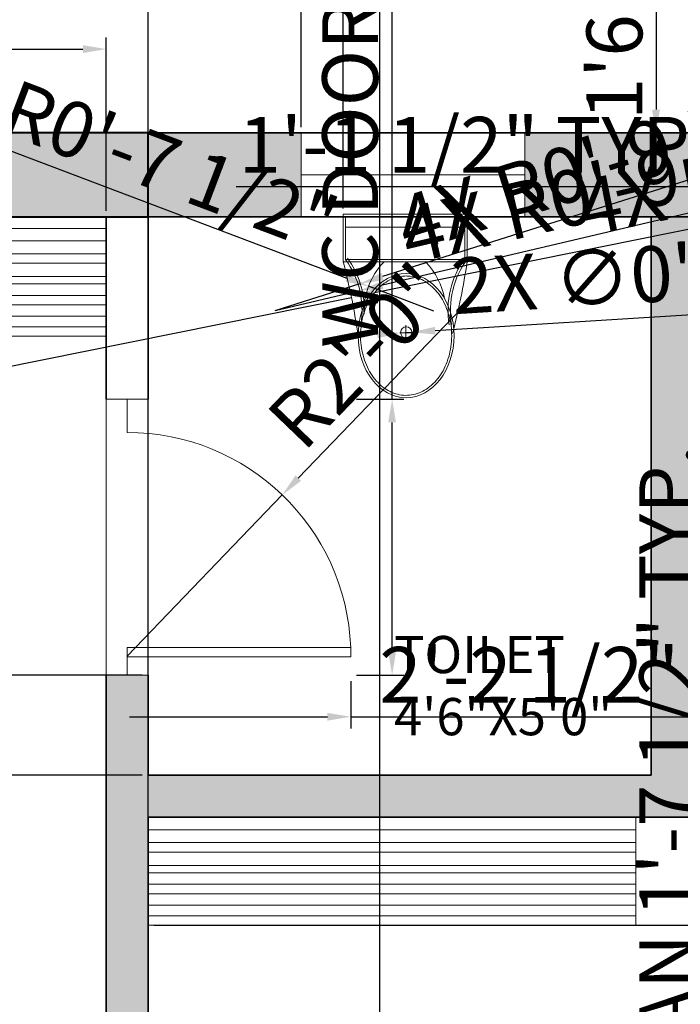
# Model space of a CAD drawing. Units: inches. Extents: x 2656 to 9931, y 1941 to 3068.
# Tile 22 of 46: x 2863 to 2934, y 2530 to 2636. Entities that reach past the tile are written whole.
import ezdxf

# ---------------------------------------------------------------- set-up
doc = ezdxf.new("R2010")
doc.units = ezdxf.units.IN
for name, color, linetype, lineweight in [('A-ANNO-DIMS', 2, 'Continuous', 18), ('A-AREA-IDEN', 7, 'Continuous', 18), ('A-COLS', 7, 'Continuous', 40), ('A-COLS-PATT', 146, 'Continuous', 13), ('A-DOOR', 3, 'Continuous', 18), ('A-FLOR-CASE', 32, 'Continuous', 18), ('A-FLOR-FIXT', 9, 'Continuous', 18), ('A-GLAZ', 4, 'Continuous', 18), ('A-WALL', 7, 'Continuous', 35), ('A-WALL-PATT', 251, 'Continuous', 13)]:
    doc.layers.add(name, color=color, linetype=linetype, lineweight=lineweight)
doc.styles.get("Standard").update_dxf_attribs({"font": 'arial.ttf'})
doc.dimstyles.new('ISO-25', dxfattribs={"dimtxt": 6, "dimasz": 2.5, "dimexe": 1.25, "dimexo": 0.625, "dimtad": 1, "dimdec": 0, "dimlunit": 3, "dimtxsty": 'Standard', "dimcen": 2.5, "dimadec": 0, "dimazin": 0, "dimtfac": 1, "dimtdec": 0, "dimtmove": 0, "dimatfit": 3, "dimfxl": 1, "dimarcsym": 0})

# ---------------------------------------------------------------- blocks, each defined once
blk = doc.blocks.new('*D2')
at = {"layer": 'A-ANNO-DIMS', "color": 0, "lineweight": -2, "transparency": 16777216}
for p, q in [((2931.82, 2641.6), (2932.44, 2641.6)), ((2931.19, 2639.1), (2931.19, 2626.1)), ((2931.82, 2623.6), (2932.44, 2623.6))]:
    blk.add_line(p, q, dxfattribs=at)
at = {"layer": 'A-ANNO-DIMS', "color": 0, "transparency": 16777216}
for points in [[(2930.77, 2639.1), (2931.61, 2639.1), (2931.19, 2641.6)], [(2930.77, 2626.1), (2931.61, 2626.1), (2931.19, 2623.6)]]:
    blk.add_solid(points, dxfattribs=at)
at = {"layer": 'Defpoints', "color": 0, "transparency": 16777216}
for p in [(2931.19, 2641.6), (2931.19, 2623.6), (2931.19, 2623.6)]:
    blk.add_point(p, dxfattribs=at)
at = {"layer": 'A-ANNO-DIMS', "color": 0, "transparency": 16777216, "insert": (2927.5, 2632.6), "char_height": 6, "attachment_point": 5, "rotation": 90}
blk.add_mtext('1\'6"', dxfattribs=at)
blk = doc.blocks.new('A$C31115884')
for p, q in [((283.1, 497.7), (223.4, 497.7)), ((257.5, 466.4), (257.5, 523.2)), ((0, 200), (0, 0)), ((520, 200), (0, 200)), ((10, 190), (10, 10)), ((510, 190), (10, 190)), ((510, 10), (510, 190)), ((520, 0), (520, 200)), ((510, 54.5), (0, 54.5)), ((10, 10), (510, 10)), ((0, 0), (520, 0))]:
    blk.add_line(p, q)
blk.add_circle((255.6, 496.4), 23.6)
for centre, radius, start, end in [((2777.7, -204.6), 2807, 165.4549, 171.7133), ((3237, 905), 2807, 188.2867, 194.5451), ((-294.5, 403.3), 364.7, 324.2091, 9.3499), ((-294.5, 403.3), 374.7, 324.2091, 9.3499), ((805.8, 403.3), 364.7, 170.6501, 215.7909), ((139.5, 406.2), 293.5, 315.8436, 2.6563), ((805.8, 403.3), 374.7, 179.2036, 215.7909), ((383.6, 406.2), 293.5, 190.2774, 224.1564)]:
    blk.add_arc(centre, radius, start, end)
blk.add_ellipse((256.2, 509.9), major_axis=(0, -260.7), ratio=0.772727)
blk.add_open_spline([(256.2, 259.2), (263.1, 259.2), (270, 259.7), (287.8, 262.3), (298.7, 265.1), (319.9, 273.1), (330.2, 278.4), (350.1, 291.1), (359.7, 298.7), (377.7, 315.9), (386.2, 325.5), (401.7, 346.6), (408.8, 358.1), (421.3, 382.5), (426.8, 395.5), (435.9, 422.4), (439.5, 436.4), (444.8, 465.1), (446.5, 479.7), (447.9, 509.2), (447.6, 524), (445, 553.3), (442.7, 567.8), (436.3, 596), (432.1, 609.7), (421.9, 636), (416, 648.6), (402.5, 672.1), (395, 683), (378.6, 703), (369.8, 712.1), (351.1, 728), (341.3, 734.8), (320.9, 746.2), (310.4, 750.7), (288.9, 757.3), (278, 759.4), (256, 761), (245, 760.6), (223.1, 757.2), (212.3, 754.3), (191.1, 746.1), (180.8, 740.7), (160.9, 727.8), (151.4, 720.1), (133.5, 702.7), (125.1, 693), (109.6, 671.7), (102.6, 660.2), (90.2, 635.7), (84.9, 622.7), (76, 595.6), (72.4, 581.6), (67.2, 552.9), (65.6, 538.2), (64.4, 508.8), (64.8, 494), (67.5, 464.7), (69.9, 450.2), (76.6, 422), (80.8, 408.3), (91.1, 382.2), (97.2, 369.7), (110.8, 346.3), (118.4, 335.4), (134.8, 315.6), (143.7, 306.7), (162.4, 290.9), (172.3, 284.2), (192.8, 273), (203.3, 268.6), (224.8, 262.2), (235.8, 260.2), (249.9, 259.3), (253, 259.2), (256.2, 259.2)], degree=3, knots=[0, 0, 0, 0, 0.110105, 0.110105, 0.285049, 0.285049, 0.459994, 0.459994, 0.634938, 0.634938, 0.809882, 0.809882, 0.984827, 0.984827, 1.159771, 1.159771, 1.334715, 1.334715, 1.50966, 1.50966, 1.684604, 1.684604, 1.859549, 1.859549, 2.034493, 2.034493, 2.209437, 2.209437, 2.384382, 2.384382, 2.559326, 2.559326, 2.73427, 2.73427, 2.909215, 2.909215, 3.084159, 3.084159, 3.259103, 3.259103, 3.434048, 3.434048, 3.608992, 3.608992, 3.783936, 3.783936, 3.958881, 3.958881, 4.133825, 4.133825, 4.30877, 4.30877, 4.483714, 4.483714, 4.658658, 4.658658, 4.833603, 4.833603, 5.008547, 5.008547, 5.183491, 5.183491, 5.358436, 5.358436, 5.53338, 5.53338, 5.708324, 5.708324, 5.883269, 5.883269, 6.058213, 6.058213, 6.233158, 6.233158, 6.283185, 6.283185, 6.283185, 6.283185])
blk = doc.blocks.new('DOOR-WC-SIDE')
for p, q in [((-0.04, 29.7), (-0.04, 0.04)), ((2.21, 29.7), (2.21, 28.12)), ((2.21, 28.12), (2.21, 26.12)), ((26.21, 3.04), (2.21, 3.04)), ((2.21, 3.04), (2.21, 2.04)), ((26.21, 2.04), (26.21, 3.04)), ((2.21, 0.04), (2.21, 2.04)), ((2.21, 2.04), (2.21, 2.04)), ((2.21, 2.04), (26.21, 2.04))]:
    blk.add_line(p, q)
blk.add_arc((2.21, 2.11), 24.02, 2.2244, 90)
blk = doc.blocks.new('WIN-VENT-24IN')
for p, q in [((23.99, 0), (23.99, 4.5)), ((-0.01, 0), (23.99, 0))]:
    blk.add_line(p, q)
blk = doc.blocks.new('WARDROBE-LONG')
for p, q in [((34.19, 12.8), (34.19, -0.03)), ((34.19, 11.55), (119.96, 11.55)), ((34.19, 10.19), (119.96, 10.19)), ((34.19, 8.82), (119.96, 8.82)), ((34.19, 7.81), (119.96, 7.81)), ((34.19, 6.39), (119.96, 6.39)), ((34.19, 5.58), (119.96, 5.58)), ((34.19, 4.35), (119.96, 4.35)), ((34.19, 3.33), (119.96, 3.33)), ((34.19, 2.12), (119.96, 2.12)), ((34.19, 2.12), (119.96, 2.12)), ((34.19, -0.03), (34.19, 0.97)), ((34.19, 0.97), (119.96, 0.97)), ((-0.04, -0.03), (119.96, -0.03))]:
    blk.add_line(p, q)
blk = doc.blocks.new('WARDROBE-SHORT')
for p, q in [((52.34, 11.6), (52.34, 0.02)), ((-0.04, 10.24), (52.34, 10.24)), ((-0.04, 8.87), (52.34, 8.87)), ((-0.04, 7.85), (52.34, 7.85)), ((-0.04, 6.43), (52.34, 6.43)), ((-0.04, 5.63), (52.34, 5.63)), ((-0.04, 4.4), (52.34, 4.4)), ((-0.04, 3.38), (52.34, 3.38)), ((-0.04, 2.17), (52.34, 2.17)), ((-0.04, 2.17), (52.34, 2.17)), ((-0.04, 1.02), (52.34, 1.02)), ((-0.04, 0.02), (52.34, 0.02))]:
    blk.add_line(p, q)
blk = doc.blocks.new('*D29')
at = {"layer": 'A-ANNO-DIMS', "color": 0, "lineweight": -2, "transparency": 16777216}
for p, q in [((2939.24, 2614.86), (2935.66, 2614.86)), ((2936.91, 2612.36), (2936.91, 2597.65)), ((2939.24, 2595.15), (2935.66, 2595.15)), ((2936.91, 2595.15), (2936.91, 2504.75))]:
    blk.add_line(p, q, dxfattribs=at)
at = {"layer": 'A-ANNO-DIMS', "color": 0, "transparency": 16777216}
for points in [[(2936.49, 2612.36), (2937.33, 2612.36), (2936.91, 2614.86)], [(2936.49, 2597.65), (2937.33, 2597.65), (2936.91, 2595.15)]]:
    blk.add_solid(points, dxfattribs=at)
at = {"layer": 'Defpoints', "color": 0, "transparency": 16777216}
for p in [(2939.87, 2614.86), (2936.91, 2595.15), (2939.87, 2595.15)]:
    blk.add_point(p, dxfattribs=at)
at = {"layer": 'A-ANNO-DIMS', "color": 0, "transparency": 16777216, "insert": (2933.18, 2548.7), "char_height": 6, "attachment_point": 5, "rotation": 90}
blk.add_mtext('WC PAN 1\'-7 1/2" TYP.', dxfattribs=at)
blk = doc.blocks.new('*D30')
at = {"layer": 'A-ANNO-DIMS', "color": 0, "lineweight": -2, "transparency": 16777216}
for p, q in [((2939.87, 2615.48), (2939.87, 2619.06)), ((2953.16, 2615.48), (2953.16, 2619.06)), ((2939.87, 2617.81), (2886.13, 2617.81)), ((2950.66, 2617.81), (2942.37, 2617.81))]:
    blk.add_line(p, q, dxfattribs=at)
at = {"layer": 'A-ANNO-DIMS', "color": 0, "transparency": 16777216}
for points in [[(2942.37, 2618.23), (2942.37, 2617.39), (2939.87, 2617.81)], [(2950.66, 2618.23), (2950.66, 2617.39), (2953.16, 2617.81)]]:
    blk.add_solid(points, dxfattribs=at)
at = {"layer": 'Defpoints', "color": 0, "transparency": 16777216}
for p in [(2939.87, 2617.81), (2939.87, 2614.86), (2953.16, 2614.86)]:
    blk.add_point(p, dxfattribs=at)
at = {"layer": 'A-ANNO-DIMS', "color": 0, "transparency": 16777216, "insert": (2911.75, 2621.54), "char_height": 6, "attachment_point": 5}
blk.add_mtext('1\'-1 1/2" TYP.', dxfattribs=at)
blk = doc.blocks.new('*D32')
at = {"layer": 'A-ANNO-DIMS', "color": 0, "lineweight": -2, "transparency": 16777216}
for p, q in [((2842.61, 2565.21), (2856.53, 2565.21)), ((2855.28, 2505.27), (2855.28, 2562.71)), ((2842.61, 2502.77), (2856.53, 2502.77))]:
    blk.add_line(p, q, dxfattribs=at)
at = {"layer": 'A-ANNO-DIMS', "color": 0, "transparency": 16777216}
for points in [[(2854.86, 2562.71), (2855.69, 2562.71), (2855.28, 2565.21)], [(2854.86, 2505.27), (2855.69, 2505.27), (2855.28, 2502.77)]]:
    blk.add_solid(points, dxfattribs=at)
at = {"layer": 'Defpoints', "color": 0, "transparency": 16777216}
for p in [(2841.98, 2565.21), (2855.28, 2565.21), (2841.98, 2502.77)]:
    blk.add_point(p, dxfattribs=at)
at = {"layer": 'A-ANNO-DIMS', "color": 0, "transparency": 16777216, "insert": (2851.55, 2533.99), "char_height": 6, "attachment_point": 5, "rotation": 90}
blk.add_mtext('5\'-2 1/2" TYP.', dxfattribs=at)
blk = doc.blocks.new('*D33')
at = {"layer": 'A-ANNO-DIMS', "color": 0, "lineweight": -2, "transparency": 16777216}
for p, q in [((2902.86, 2595), (2902.86, 2693.32)), ((2899.03, 2595), (2904.11, 2595)), ((2902.86, 2567.84), (2902.86, 2592.5)), ((2899.03, 2565.34), (2904.11, 2565.34))]:
    blk.add_line(p, q, dxfattribs=at)
at = {"layer": 'A-ANNO-DIMS', "color": 0, "transparency": 16777216}
for points in [[(2902.44, 2592.5), (2903.27, 2592.5), (2902.86, 2595)], [(2902.44, 2567.84), (2903.27, 2567.84), (2902.86, 2565.34)]]:
    blk.add_solid(points, dxfattribs=at)
at = {"layer": 'Defpoints', "color": 0, "transparency": 16777216}
for p in [(2898.41, 2595), (2902.86, 2595), (2898.41, 2565.34)]:
    blk.add_point(p, dxfattribs=at)
at = {"layer": 'A-ANNO-DIMS', "color": 0, "transparency": 16777216, "insert": (2899.13, 2645.41), "char_height": 6, "attachment_point": 5, "rotation": 90}
blk.add_mtext('WC DOOR 2\'-5 1/2" TYP.', dxfattribs=at)
blk = doc.blocks.new('*D34')
at = {"layer": 'A-ANNO-DIMS', "color": 0, "lineweight": -2, "transparency": 16777216}
for p, q in [((2872.16, 2564.71), (2872.16, 2559.64)), ((2898.41, 2564.71), (2898.41, 2559.64)), ((2874.66, 2560.89), (2895.91, 2560.89)), ((2898.41, 2560.89), (2952.81, 2560.89))]:
    blk.add_line(p, q, dxfattribs=at)
at = {"layer": 'A-ANNO-DIMS', "color": 0, "transparency": 16777216}
for points in [[(2874.66, 2561.3), (2874.66, 2560.47), (2872.16, 2560.89)], [(2895.91, 2561.3), (2895.91, 2560.47), (2898.41, 2560.89)]]:
    blk.add_solid(points, dxfattribs=at)
at = {"layer": 'Defpoints', "color": 0, "transparency": 16777216}
for p in [(2872.16, 2565.34), (2898.41, 2565.34), (2898.41, 2560.89)]:
    blk.add_point(p, dxfattribs=at)
at = {"layer": 'A-ANNO-DIMS', "color": 0, "transparency": 16777216, "insert": (2926.86, 2564.61), "char_height": 6, "attachment_point": 5}
blk.add_mtext('2\'-2 1/2" TYP.', dxfattribs=at)
blk = doc.blocks.new('*D57')
at = {"layer": 'A-ANNO-DIMS', "color": 0, "lineweight": -2, "transparency": 16777216}
for p, q in [((2752.16, 2615.23), (2752.16, 2633.85)), ((2872.16, 2615.23), (2872.16, 2633.85)), ((2754.66, 2632.6), (2869.66, 2632.6))]:
    blk.add_line(p, q, dxfattribs=at)
at = {"layer": 'A-ANNO-DIMS', "color": 0, "transparency": 16777216}
for points in [[(2754.66, 2633.02), (2754.66, 2632.18), (2752.16, 2632.6)], [(2869.66, 2633.02), (2869.66, 2632.18), (2872.16, 2632.6)]]:
    blk.add_solid(points, dxfattribs=at)
at = {"layer": 'Defpoints', "color": 0, "transparency": 16777216}
for p in [(2872.16, 2632.6), (2752.16, 2614.6), (2872.16, 2614.6)]:
    blk.add_point(p, dxfattribs=at)
at = {"layer": 'A-ANNO-DIMS', "color": 0, "transparency": 16777216, "insert": (2812.16, 2636.33), "char_height": 6, "attachment_point": 5}
blk.add_mtext('WARDROBE 10\'-0" TYP.', dxfattribs=at)
blk = doc.blocks.new('*D98')
at = {"layer": 'A-ANNO-DIMS', "color": 0, "lineweight": -2, "transparency": 16777216}
for p, q in [((2876.66, 2624.23), (2876.66, 2674.45)), ((2893.09, 2624.23), (2893.09, 2674.45)), ((2879.16, 2673.2), (2890.59, 2673.2)), ((2893.09, 2673.2), (2926.2, 2673.2))]:
    blk.add_line(p, q, dxfattribs=at)
at = {"layer": 'A-ANNO-DIMS', "color": 0, "transparency": 16777216}
for points in [[(2879.16, 2673.62), (2879.16, 2672.78), (2876.66, 2673.2)], [(2890.59, 2673.62), (2890.59, 2672.78), (2893.09, 2673.2)]]:
    blk.add_solid(points, dxfattribs=at)
at = {"layer": 'Defpoints', "color": 0, "transparency": 16777216}
for p in [(2893.09, 2673.2), (2876.66, 2623.6), (2893.09, 2623.6)]:
    blk.add_point(p, dxfattribs=at)
at = {"layer": 'A-ANNO-DIMS', "color": 0, "transparency": 16777216, "insert": (2910.89, 2676.93), "char_height": 6, "attachment_point": 5}
blk.add_mtext('1\'-4 1/2"', dxfattribs=at)
blk = doc.blocks.new('*D100')
at = {"layer": 'A-ANNO-DIMS', "color": 0, "lineweight": -2, "transparency": 16777216}
for p, q in [((2696.56, 2565.34), (2696.56, 2603.68)), ((2876.03, 2565.34), (2695.31, 2565.34)), ((2696.56, 2557.1), (2696.56, 2562.84)), ((2876.03, 2554.6), (2695.31, 2554.6))]:
    blk.add_line(p, q, dxfattribs=at)
at = {"layer": 'A-ANNO-DIMS', "color": 0, "transparency": 16777216}
for points in [[(2696.14, 2562.84), (2696.97, 2562.84), (2696.56, 2565.34)], [(2696.14, 2557.1), (2696.97, 2557.1), (2696.56, 2554.6)]]:
    blk.add_solid(points, dxfattribs=at)
at = {"layer": 'Defpoints', "color": 0, "transparency": 16777216}
for p in [(2696.56, 2565.34), (2876.66, 2565.34), (2876.66, 2554.6)]:
    blk.add_point(p, dxfattribs=at)
at = {"layer": 'A-ANNO-DIMS', "color": 0, "transparency": 16777216, "insert": (2692.83, 2585.76), "char_height": 6, "attachment_point": 5, "rotation": 90}
blk.add_mtext('0\'-10 1/2"', dxfattribs=at)
blk = doc.blocks.new('*D102')
at = {"layer": 'A-ANNO-DIMS', "color": 0, "lineweight": -2, "transparency": 16777216}
for p, q in [((2998.16, 2604.98), (2998.16, 2009.27)), ((2872.16, 2564.71), (2872.16, 2009.27)), ((2874.66, 2010.52), (2995.66, 2010.52))]:
    blk.add_line(p, q, dxfattribs=at)
at = {"layer": 'A-ANNO-DIMS', "color": 0, "transparency": 16777216}
for points in [[(2874.66, 2010.94), (2874.66, 2010.11), (2872.16, 2010.52)], [(2995.66, 2010.94), (2995.66, 2010.11), (2998.16, 2010.52)]]:
    blk.add_solid(points, dxfattribs=at)
at = {"layer": 'Defpoints', "color": 0, "transparency": 16777216}
for p in [(2998.16, 2605.6), (2872.16, 2565.34), (2998.16, 2010.52)]:
    blk.add_point(p, dxfattribs=at)
at = {"layer": 'A-ANNO-DIMS', "color": 0, "transparency": 16777216, "insert": (2935.16, 2014.21), "char_height": 6, "attachment_point": 5}
blk.add_mtext('10\'-6"', dxfattribs=at)
blk = doc.blocks.new('*D130')
at = {"layer": 'A-ANNO-DIMS', "color": 0, "lineweight": -2, "transparency": 16777216}
for p, q in [((2877.28, 2538.52), (3061.01, 2538.52)), ((3059.76, 2536.02), (3059.76, 2525.32)), ((2902.17, 2522.82), (3061.01, 2522.82)), ((3059.76, 2522.82), (3059.76, 2489.7))]:
    blk.add_line(p, q, dxfattribs=at)
at = {"layer": 'A-ANNO-DIMS', "color": 0, "transparency": 16777216}
for points in [[(3059.34, 2536.02), (3060.17, 2536.02), (3059.76, 2538.52)], [(3059.34, 2525.32), (3060.17, 2525.32), (3059.76, 2522.82)]]:
    blk.add_solid(points, dxfattribs=at)
at = {"layer": 'Defpoints', "color": 0, "transparency": 16777216}
for p in [(2876.66, 2538.52), (2901.54, 2522.82), (3059.76, 2522.82)]:
    blk.add_point(p, dxfattribs=at)
at = {"layer": 'A-ANNO-DIMS', "color": 0, "transparency": 16777216, "insert": (3056.03, 2505.01), "char_height": 6, "attachment_point": 5, "rotation": 90}
blk.add_mtext('1\'-3 1/2"', dxfattribs=at)
blk = doc.blocks.new('*D131')
at = {"layer": 'A-ANNO-DIMS', "color": 0, "lineweight": -2, "transparency": 16777216}
for p, q in [((2876.66, 2539.14), (2876.66, 2674.45)), ((2901.54, 2523.44), (2901.54, 2674.45)), ((2879.16, 2673.2), (2899.04, 2673.2))]:
    blk.add_line(p, q, dxfattribs=at)
at = {"layer": 'A-ANNO-DIMS', "color": 0, "transparency": 16777216}
for points in [[(2879.16, 2673.62), (2879.16, 2672.78), (2876.66, 2673.2)], [(2899.04, 2673.62), (2899.04, 2672.78), (2901.54, 2673.2)]]:
    blk.add_solid(points, dxfattribs=at)
at = {"layer": 'Defpoints', "color": 0, "transparency": 16777216}
for p in [(2901.54, 2673.2), (2876.66, 2538.52), (2901.54, 2522.82)]:
    blk.add_point(p, dxfattribs=at)
at = {"layer": 'A-ANNO-DIMS', "color": 0, "transparency": 16777216, "insert": (2889.1, 2676.84), "char_height": 6, "attachment_point": 5}
blk.add_mtext('2\'-1"', dxfattribs=at)
blk = doc.blocks.new('*D174')
at = {"layer": 'A-ANNO-DIMS', "color": 0, "lineweight": -2, "transparency": 16777216}
for p, q in [((2743.16, 2624.23), (2743.16, 2674.45)), ((2998.16, 2624.23), (2998.16, 2674.45)), ((2745.66, 2673.2), (2995.66, 2673.2))]:
    blk.add_line(p, q, dxfattribs=at)
at = {"layer": 'A-ANNO-DIMS', "color": 0, "transparency": 16777216}
for points in [[(2745.66, 2673.62), (2745.66, 2672.78), (2743.16, 2673.2)], [(2995.66, 2673.62), (2995.66, 2672.78), (2998.16, 2673.2)]]:
    blk.add_solid(points, dxfattribs=at)
at = {"layer": 'Defpoints', "color": 0, "transparency": 16777216}
for p in [(2998.16, 2673.2), (2743.16, 2623.6), (2998.16, 2623.6)]:
    blk.add_point(p, dxfattribs=at)
at = {"layer": 'A-ANNO-DIMS', "color": 0, "transparency": 16777216, "insert": (2870.66, 2676.89), "char_height": 6, "attachment_point": 5}
blk.add_mtext('21\'-3"', dxfattribs=at)
blk = doc.blocks.new('*D176')
at = {"layer": 'A-ANNO-DIMS', "color": 0, "lineweight": -2, "transparency": 16777216}
for p, q in [((2876.66, 2615.23), (2876.66, 2674.45)), ((2897.62, 2615.48), (2897.62, 2674.45)), ((2879.16, 2673.2), (2895.12, 2673.2))]:
    blk.add_line(p, q, dxfattribs=at)
at = {"layer": 'A-ANNO-DIMS', "color": 0, "transparency": 16777216}
for points in [[(2879.16, 2673.62), (2879.16, 2672.78), (2876.66, 2673.2)], [(2895.12, 2673.62), (2895.12, 2672.78), (2897.62, 2673.2)]]:
    blk.add_solid(points, dxfattribs=at)
at = {"layer": 'Defpoints', "color": 0, "transparency": 16777216}
for p in [(2897.62, 2673.2), (2876.66, 2614.6), (2897.62, 2614.86)]:
    blk.add_point(p, dxfattribs=at)
at = {"layer": 'A-ANNO-DIMS', "color": 0, "transparency": 16777216, "insert": (2887.14, 2676.89), "char_height": 6, "attachment_point": 5}
blk.add_mtext('1\'-9"', dxfattribs=at)
blk = doc.blocks.new('*D177')
at = {"layer": 'A-ANNO-DIMS', "color": 0, "lineweight": -2, "transparency": 16777216}
for p, q in [((2935.16, 2615.23), (2935.16, 2674.45)), ((2939.87, 2615.48), (2939.87, 2674.45)), ((2932.66, 2673.2), (2930.16, 2673.2)), ((2935.16, 2673.2), (2939.87, 2673.2)), ((2942.37, 2673.2), (2976.05, 2673.2))]:
    blk.add_line(p, q, dxfattribs=at)
at = {"layer": 'A-ANNO-DIMS', "color": 0, "transparency": 16777216}
for points in [[(2932.66, 2673.62), (2932.66, 2672.78), (2935.16, 2673.2)], [(2942.37, 2673.62), (2942.37, 2672.78), (2939.87, 2673.2)]]:
    blk.add_solid(points, dxfattribs=at)
at = {"layer": 'Defpoints', "color": 0, "transparency": 16777216}
for p in [(2939.87, 2673.2), (2935.16, 2614.6), (2939.87, 2614.86)]:
    blk.add_point(p, dxfattribs=at)
at = {"layer": 'A-ANNO-DIMS', "color": 0, "transparency": 16777216, "insert": (2960.46, 2676.93), "char_height": 6, "attachment_point": 5}
blk.add_mtext('0\'-4 1/2"', dxfattribs=at)
blk = doc.blocks.new('*D186')
at = {"layer": 'A-ANNO-DIMS', "color": 0, "lineweight": -2, "transparency": 16777216}
for p, q in [((2910.43, 2604.85), (2892.79, 2586.52)), ((2874.41, 2567.41), (2891.06, 2584.71))]:
    blk.add_line(p, q, dxfattribs=at)
at = {"layer": 'A-ANNO-DIMS', "color": 0, "transparency": 16777216}
blk.add_solid([(2892.49, 2586.81), (2893.09, 2586.23), (2891.06, 2584.71)], dxfattribs=at)
at = {"layer": 'Defpoints', "color": 0, "transparency": 16777216}
for p in [(2891.06, 2584.71), (2874.41, 2567.41)]:
    blk.add_point(p, dxfattribs=at)
at = {"layer": 'A-ANNO-DIMS', "color": 0, "transparency": 16777216, "insert": (2899.82, 2599.14), "char_height": 6, "attachment_point": 5, "rotation": 46.112}
blk.add_mtext('R2\'-0"', dxfattribs=at)
blk = doc.blocks.new('*D189')
at = {"layer": 'A-ANNO-DIMS', "color": 0, "lineweight": -2, "transparency": 16777216}
for p, q in [((2958.39, 2618.02), (2900.95, 2606.42)), ((2828.14, 2591.72), (2898.5, 2605.92))]:
    blk.add_line(p, q, dxfattribs=at)
at = {"layer": 'A-ANNO-DIMS', "color": 0, "transparency": 16777216}
blk.add_solid([(2900.86, 2606.83), (2901.03, 2606.01), (2898.5, 2605.92)], dxfattribs=at)
at = {"layer": 'Defpoints', "color": 0, "transparency": 16777216}
for p in [(2898.5, 2605.92), (2828.14, 2591.72)]:
    blk.add_point(p, dxfattribs=at)
at = {"layer": 'A-ANNO-DIMS', "color": 0, "transparency": 16777216, "insert": (2939.98, 2618.06), "char_height": 6, "attachment_point": 5, "rotation": 11.4157}
blk.add_mtext('4X R6\'-0"', dxfattribs=at)
blk = doc.blocks.new('*D190')
at = {"layer": 'A-ANNO-DIMS', "color": 0, "lineweight": -2, "transparency": 16777216}
for p, q in [((2951.95, 2623.98), (2901.83, 2608.18)), ((2890.31, 2604.54), (2899.44, 2607.42))]:
    blk.add_line(p, q, dxfattribs=at)
at = {"layer": 'A-ANNO-DIMS', "color": 0, "transparency": 16777216}
blk.add_solid([(2901.7, 2608.57), (2901.95, 2607.78), (2899.44, 2607.42)], dxfattribs=at)
at = {"layer": 'Defpoints', "color": 0, "transparency": 16777216}
for p in [(2899.44, 2607.42), (2890.31, 2604.54)]:
    blk.add_point(p, dxfattribs=at)
at = {"layer": 'A-ANNO-DIMS', "color": 0, "transparency": 16777216, "insert": (2926.96, 2620.01), "char_height": 6, "attachment_point": 5, "rotation": 17.4987}
blk.add_mtext('4X R0\'-9 1/2"', dxfattribs=at)
blk = doc.blocks.new('*D191')
at = {"layer": 'A-ANNO-DIMS', "color": 0, "lineweight": -2, "transparency": 16777216}
for p, q in [((2952.98, 2619.27), (2901.82, 2607.25)), ((2890.31, 2604.54), (2899.39, 2606.68))]:
    blk.add_line(p, q, dxfattribs=at)
at = {"layer": 'A-ANNO-DIMS', "color": 0, "transparency": 16777216}
blk.add_solid([(2901.72, 2607.65), (2901.91, 2606.84), (2899.39, 2606.68)], dxfattribs=at)
at = {"layer": 'Defpoints', "color": 0, "transparency": 16777216}
for p in [(2899.39, 2606.68), (2890.31, 2604.54)]:
    blk.add_point(p, dxfattribs=at)
at = {"layer": 'A-ANNO-DIMS', "color": 0, "transparency": 16777216, "insert": (2927.76, 2617.17), "char_height": 6, "attachment_point": 5, "rotation": 13.2221}
blk.add_mtext('4X R0\'-9 1/2"', dxfattribs=at)
blk = doc.blocks.new('*D192')
at = {"layer": 'A-ANNO-DIMS', "color": 0, "lineweight": -2, "transparency": 16777216}
for p, q in [((2848.84, 2626.63), (2897.99, 2608.01)), ((2907.35, 2604.47), (2900.33, 2607.13))]:
    blk.add_line(p, q, dxfattribs=at)
at = {"layer": 'A-ANNO-DIMS', "color": 0, "transparency": 16777216}
blk.add_solid([(2898.14, 2608.4), (2897.84, 2607.62), (2900.33, 2607.13)], dxfattribs=at)
at = {"layer": 'Defpoints', "color": 0, "transparency": 16777216}
for p in [(2900.33, 2607.13), (2907.35, 2604.47)]:
    blk.add_point(p, dxfattribs=at)
at = {"layer": 'A-ANNO-DIMS', "color": 0, "transparency": 16777216, "insert": (2873.57, 2621.25), "char_height": 6, "attachment_point": 5, "rotation": 339.2505}
blk.add_mtext('4X R0\'-7 1/2"', dxfattribs=at)
blk = doc.blocks.new('*D193')
at = {"layer": 'A-ANNO-DIMS', "color": 0, "lineweight": -2, "transparency": 16777216}
for p, q in [((2946.3, 2604.75), (2907.47, 2602.35)), ((2901.28, 2601.97), (2898.78, 2601.82)), ((2903.77, 2602.12), (2904.98, 2602.2))]:
    blk.add_line(p, q, dxfattribs=at)
at = {"layer": 'A-ANNO-DIMS', "color": 0, "transparency": 16777216}
for points in [[(2907.45, 2602.77), (2907.5, 2601.94), (2904.98, 2602.2)], [(2901.25, 2602.39), (2901.3, 2601.55), (2903.77, 2602.12)]]:
    blk.add_solid(points, dxfattribs=at)
at = {"layer": 'Defpoints', "color": 0, "transparency": 16777216}
for p in [(2903.77, 2602.12), (2904.98, 2602.2)]:
    blk.add_point(p, dxfattribs=at)
at = {"layer": 'A-ANNO-DIMS', "color": 0, "transparency": 16777216, "insert": (2927.9, 2607.48), "char_height": 6, "attachment_point": 5, "rotation": 3.5337}
blk.add_mtext('2X ∅0\'-1"', dxfattribs=at)

msp = doc.modelspace()

# ---------------------------------------------------------------- hatches: boundary and pattern name
at = {"layer": 'A-COLS-PATT'}
h = msp.add_hatch(color=256, dxfattribs=at)
h.dxf.hatch_style = 1
h.paths.add_polyline_path([(2752.16, 2623.6), (2743.16, 2623.6), (2743.16, 2605.6), (2752.16, 2605.6)])
h.paths.add_polyline_path([(2876.66, 2623.6), (2858.66, 2623.6), (2858.66, 2614.6), (2876.66, 2614.6)])
h.paths.add_polyline_path([(2998.16, 2623.6), (2989.16, 2623.6), (2989.16, 2614.6), (2989.16, 2605.6), (2998.16, 2605.6)])
h.paths.add_polyline_path([(2998.16, 2444.1), (2989.16, 2444.1), (2989.16, 2426.1), (2998.16, 2426.1)])
h.paths.add_polyline_path([(2876.66, 2444.1), (2867.66, 2444.1), (2867.66, 2426.1), (2876.66, 2426.1)])
h.paths.add_polyline_path([(2752.16, 2444.1), (2743.16, 2444.1), (2743.16, 2426.1), (2752.16, 2426.1)])
h.paths.add_polyline_path([(2752.16, 2300.1), (2743.16, 2300.1), (2743.16, 2282.1), (2752.16, 2282.1)])
h.paths.add_polyline_path([(2876.66, 2300.1), (2867.66, 2300.1), (2867.66, 2282.1), (2876.66, 2282.1)])
h.paths.add_polyline_path([(2998.16, 2300.1), (2989.16, 2300.1), (2989.16, 2282.1), (2998.16, 2282.1)])
h.paths.add_polyline_path([(2998.16, 2184.6), (2989.16, 2184.6), (2989.16, 2166.6), (2998.16, 2166.6)])
h.paths.add_polyline_path([(2876.66, 2175.6), (2858.66, 2175.6), (2858.66, 2166.6), (2876.66, 2166.6)])
h.paths.add_polyline_path([(2752.16, 2184.6), (2743.16, 2184.6), (2743.16, 2166.6), (2752.16, 2166.6)])
at = {"layer": 'A-WALL-PATT'}
h = msp.add_hatch(color=256, dxfattribs=at)
h.dxf.hatch_style = 1
h.paths.add_polyline_path([(2858.66, 2623.6), (2752.16, 2623.6), (2752.16, 2614.6), (2858.66, 2614.6)])
h.paths.add_polyline_path([(2893.09, 2623.6), (2876.66, 2623.6), (2876.66, 2614.6), (2893.09, 2614.6), (2893.09, 2619.1)])
h.paths.add_polyline_path([(2946.51, 2623.6), (2917.09, 2623.6), (2917.09, 2614.6), (2946.51, 2614.6), (2946.51, 2619.1)])
h.paths.add_polyline_path([(2989.16, 2623.6), (2970.51, 2623.6), (2970.51, 2614.6), (2989.16, 2614.6)])
h.paths.add_polyline_path([(2998.16, 2605.6), (2989.16, 2605.6), (2989.16, 2523.88), (2998.16, 2523.88)])
h.paths.add_polyline_path([(2935.16, 2614.6), (2930.66, 2614.6), (2930.66, 2554.6), (2876.66, 2554.6), (2876.66, 2565.34), (2872.16, 2565.34), (2872.16, 2444.1), (2876.66, 2444.1), (2876.66, 2550.1), (2946.47, 2550.1), (2946.47, 2554.6), (2935.16, 2554.6)])
h.paths.add_polyline_path([(2989.16, 2554.6), (2982.11, 2554.6), (2976.57, 2554.6), (2976.57, 2550.1), (2982.11, 2550.1), (2989.16, 2550.1)])
h.paths.add_polyline_path([(2876.66, 2614.6), (2872.16, 2614.6), (2872.16, 2595), (2876.66, 2595)], flags=0)
h.paths.add_polyline_path([(2752.16, 2605.6), (2743.16, 2605.6), (2743.16, 2544.03), (2752.16, 2544.03)])
h.paths.add_polyline_path([(2752.16, 2426.1), (2743.16, 2426.1), (2743.16, 2300.1), (2752.16, 2300.1)])
h.paths.add_polyline_path([(2821.13, 2430.6), (2752.16, 2430.6), (2752.16, 2426.1), (2821.13, 2426.1)])
h.paths.add_polyline_path([(2867.66, 2430.6), (2862.88, 2430.6), (2862.88, 2426.1), (2867.66, 2426.1)])
h.paths.add_polyline_path([(2752.16, 2484.03), (2747.66, 2484.03), (2743.16, 2484.03), (2743.16, 2444.1), (2752.16, 2444.1)])
h.paths.add_polyline_path([(2998.16, 2426.1), (2989.16, 2426.1), (2989.16, 2390.1), (2872.16, 2390.1), (2872.16, 2385.6), (2876.66, 2385.6), (2989.16, 2385.6), (2989.16, 2365.04), (2998.16, 2365.04)])
h.paths.add_polyline_path([(2998.16, 2463.88), (2993.66, 2463.88), (2989.16, 2463.88), (2989.16, 2444.1), (2998.16, 2444.1)])
h.paths.add_polyline_path([(2998.16, 2319.88), (2989.16, 2319.88), (2989.16, 2300.1), (2998.16, 2300.1)])
h.paths.add_polyline_path([(2998.16, 2282.1), (2989.16, 2282.1), (2989.16, 2253.6), (2982.06, 2253.6), (2982.06, 2249.1), (2989.16, 2249.1), (2998.16, 2249.1)])
h.paths.add_polyline_path([(2931.54, 2253.6), (2923.8, 2253.6), (2923.8, 2249.1), (2931.54, 2249.1)])
h.paths.add_polyline_path([(2876.66, 2282.1), (2872.16, 2282.1), (2872.16, 2184.6), (2872.16, 2175.6), (2876.66, 2175.6), (2876.66, 2249.1), (2888.32, 2249.1), (2888.32, 2251.35), (2888.32, 2253.6), (2876.66, 2253.6)])
h.paths.add_polyline_path([(2858.66, 2175.6), (2841.42, 2175.6), (2841.42, 2166.6), (2858.66, 2166.6)])
h.paths.add_polyline_path([(2785.06, 2171.1), (2785.06, 2175.6), (2752.16, 2175.6), (2752.16, 2166.6), (2785.06, 2166.6)])
h.paths.add_polyline_path([(2752.16, 2282.1), (2743.16, 2282.1), (2743.16, 2184.6), (2752.16, 2184.6)])
h.paths.add_polyline_path([(2809.77, 2300.1), (2752.16, 2300.1), (2752.16, 2295.6), (2809.77, 2295.6)])
h.paths.add_polyline_path([(2867.66, 2300.1), (2851.88, 2300.1), (2851.88, 2295.6), (2867.66, 2295.6)])

# ---------------------------------------------------------------- linework, layer by layer
at = {"layer": 'A-COLS'}
for p, q in [((2876.66, 2623.6), (2858.66, 2623.6)), ((2876.66, 2614.6), (2876.66, 2623.6)), ((2858.66, 2614.6), (2876.66, 2614.6))]:
    msp.add_line(p, q, dxfattribs=at)
at = {"layer": 'A-DOOR'}
for p, q in [((2872.16, 2595), (2876.66, 2595)), ((2872.16, 2565.34), (2876.66, 2565.34))]:
    msp.add_line(p, q, dxfattribs=at)
at = {"layer": 'A-GLAZ'}
for p, q in [((2893.09, 2623.6), (2893.09, 2614.6)), ((2917.09, 2623.6), (2917.09, 2614.6)), ((2893.09, 2614.6), (2893.09, 2619.1))]:
    msp.add_line(p, q, dxfattribs=at)
at = {"layer": 'A-WALL'}
for p, q in [((2743.16, 2623.6), (2998.16, 2623.6)), ((2752.16, 2614.6), (2989.16, 2614.6)), ((2872.16, 2614.6), (2872.16, 2595)), ((2876.66, 2614.6), (2876.66, 2595)), ((2930.66, 2614.6), (2930.66, 2554.6)), ((2872.16, 2565.34), (2872.16, 2444.1)), ((2876.66, 2565.34), (2876.66, 2554.6)), ((2876.66, 2554.6), (2930.66, 2554.6)), ((2876.66, 2550.1), (2876.66, 2426.1)), ((2876.66, 2550.1), (2946.47, 2550.1)), ((2876.66, 2550.1), (2962.42, 2550.1))]:
    msp.add_line(p, q, dxfattribs=at)

# ---------------------------------------------------------------- block references
at = {"layer": 'A-DOOR'}
msp.add_blockref('DOOR-WC-SIDE', (2872.2, 2565.3), dxfattribs=at)
at = {"layer": 'A-FLOR-CASE'}
for name, p in [('WARDROBE-LONG', (2752.2, 2601.8)), ('WARDROBE-SHORT', (2876.7, 2538.5))]:
    msp.add_blockref(name, p, dxfattribs=at)
at = {"layer": 'A-FLOR-FIXT', "xscale": 0.0255708354650279, "yscale": 0.0255708354650279, "zscale": 0.0255708354650279, "rotation": 180}
msp.add_blockref('A$C31115884', (2910.91, 2614.86), dxfattribs=at)
at = {"layer": 'A-GLAZ'}
msp.add_blockref('WIN-VENT-24IN', (2893.1, 2619.1), dxfattribs=at)

# ---------------------------------------------------------------- texts
at = {"layer": 'A-AREA-IDEN', "insert": (2903.06, 2576.24), "char_height": 4, "attachment_point": 1}
msp.add_mtext_dynamic_manual_height_columns('\\PTOILET\\P4\'6"X5\'0"', width=137.4726, gutter_width=12.5, heights=[0], dxfattribs=at)

# ---------------------------------------------------------------- dimensions: what is measured, and where the dimension line sits
at = {"layer": 'A-ANNO-DIMS'}
for base, p1, p2, angle, text, override, picture, middle in [((2902.86, 2595), (2898.41, 2565.34), (2898.41, 2595), 90, 'WC DOOR <> TYP.', {"dimdec": 1, "dimlfac": 1, "dimrnd": 0, "dimzin": 1, "dimdsep": 46, "dimlunit": 4, "dimfrac": 2}, '*D33', (2899.13, 2645.41)), ((2931.19, 2623.6), (2931.19, 2641.6), (2931.19, 2623.6), 90, '1\'6"', {"dimclrd": 0, "dimclre": 0, "dimclrt": 0}, '*D2', (2927.5, 2632.6)), ((2939.87, 2617.81), (2953.16, 2614.86), (2939.87, 2614.86), 180, '<> TYP.', {"dimdec": 1, "dimlfac": 1, "dimrnd": 0, "dimzin": 1, "dimdsep": 46, "dimlunit": 4, "dimfrac": 2}, '*D30', (2911.75, 2621.54)), ((2936.91, 2595.15), (2939.87, 2614.86), (2939.87, 2595.15), 270, 'WC PAN <> TYP.', {"dimdec": 1, "dimlfac": 1, "dimrnd": 0, "dimzin": 1, "dimdsep": 46, "dimlunit": 4, "dimfrac": 2}, '*D29', (2933.18, 2548.7)), ((2855.28, 2565.21), (2841.98, 2502.77), (2841.98, 2565.21), 90, '<> TYP.', {"dimdec": 1, "dimlfac": 1, "dimrnd": 0, "dimzin": 1, "dimdsep": 46, "dimlunit": 4, "dimfrac": 2}, '*D32', (2851.55, 2533.99))]:
    dim = msp.add_linear_dim(base=base, p1=p1, p2=p2, angle=angle, text=text, dimstyle='ISO-25', override=override, dxfattribs=at)
    dim.commit()
    dim.dimension.update_dxf_attribs({"geometry": picture, "text_midpoint": middle})
for base, p1, p2, picture, middle in [((2893.09, 2673.2), (2876.66, 2623.6), (2893.09, 2623.6), '*D98', (2910.89, 2676.93)), ((2939.87, 2673.2), (2935.16, 2614.6), (2939.87, 2614.86), '*D177', (2960.46, 2676.93)), ((2998.16, 2673.2), (2743.16, 2623.6), (2998.16, 2623.6), '*D174', (2870.66, 2676.89)), ((2897.62, 2673.2), (2876.66, 2614.6), (2897.62, 2614.86), '*D176', (2887.14, 2676.89)), ((2901.54, 2673.2), (2876.66, 2538.52), (2901.54, 2522.82), '*D131', (2889.1, 2676.84)), ((2998.16, 2010.52), (2872.16, 2565.34), (2998.16, 2605.6), '*D102', (2935.16, 2014.21))]:
    dim = msp.add_linear_dim(base=base, p1=p1, p2=p2, dimstyle='ISO-25', override={"dimdec": 1, "dimlfac": 1, "dimrnd": 0, "dimzin": 1, "dimdsep": 46, "dimlunit": 4, "dimfrac": 2}, dxfattribs=at)
    dim.commit()
    dim.dimension.update_dxf_attribs({"geometry": picture, "text_midpoint": middle})
for base, p1, p2, text, picture, middle in [((2872.16, 2632.6), (2752.16, 2614.6), (2872.16, 2614.6), 'WARDROBE <> TYP.', '*D57', (2812.16, 2636.33)), ((2898.40725845, 2560.88740193), (2872.15725845, 2565.33730739), (2898.40725845, 2565.33730739), '<> TYP.', '*D34', (2926.86036213, 2564.61472116))]:
    dim = msp.add_linear_dim(base=base, p1=p1, p2=p2, text=text, dimstyle='ISO-25', override={"dimdec": 1, "dimlfac": 1, "dimrnd": 0, "dimzin": 1, "dimdsep": 46, "dimlunit": 4, "dimfrac": 2}, dxfattribs=at)
    dim.commit()
    dim.dimension.update_dxf_attribs({"geometry": picture, "text_midpoint": middle})
for center, mpoint, picture, middle in [((2907.35, 2604.47), (2900.33, 2607.13), '*D192', (2873.57, 2621.25)), ((2890.31, 2604.54), (2899.44, 2607.42), '*D190', (2926.96, 2620.01)), ((2890.31, 2604.54), (2899.39, 2606.68), '*D191', (2927.76, 2617.17))]:
    dim = msp.add_radius_dim(center=center, mpoint=mpoint, text='4X <>', dimstyle='ISO-25', override={"dimdec": 1, "dimlfac": 1, "dimrnd": 0, "dimzin": 1, "dimdsep": 46, "dimlunit": 4, "dimfrac": 2}, dxfattribs=at)
    dim.commit()
    dim.dimension.update_dxf_attribs({"geometry": picture, "text_midpoint": middle})
dim = msp.add_radius_dim(center=(2828.14, 2591.72), mpoint=(2898.5, 2605.92), text='4X <>', dimstyle='ISO-25', override={"dimdec": 1, "dimlfac": 1, "dimrnd": 0, "dimzin": 1, "dimdsep": 46, "dimlunit": 4, "dimfrac": 2}, dxfattribs=at)
dim.commit()
dim.dimension.update_dxf_attribs({"geometry": '*D189', "text_midpoint": (2940.71, 2614.45), "dimtype": 164})
dim = msp.add_diameter_dim_2p(p1=(2903.77, 2602.12), p2=(2904.98, 2602.2), text='2X <>', dimstyle='ISO-25', override={"dimdec": 1, "dimlfac": 1, "dimrnd": 0, "dimzin": 1, "dimdsep": 46, "dimlunit": 4, "dimfrac": 2}, dxfattribs=at)
dim.commit()
dim.dimension.update_dxf_attribs({"geometry": '*D193', "text_midpoint": (2928.14, 2603.63), "dimtype": 163})
dim = msp.add_radius_dim(center=(2874.41, 2567.41), mpoint=(2891.06, 2584.71), dimstyle='ISO-25', override={"dimdec": 1, "dimlfac": 1, "dimrnd": 0, "dimzin": 1, "dimdsep": 46, "dimlunit": 4, "dimfrac": 2}, dxfattribs=at)
dim.commit()
dim.dimension.update_dxf_attribs({"geometry": '*D186', "text_midpoint": (2899.82, 2599.14)})
for base, p1, p2, picture, middle in [((2696.56, 2565.34), (2876.66, 2554.6), (2876.66, 2565.34), '*D100', (2692.83, 2585.76)), ((3059.76, 2522.82), (2876.66, 2538.52), (2901.54, 2522.82), '*D130', (3056.03, 2505.01))]:
    dim = msp.add_linear_dim(base=base, p1=p1, p2=p2, angle=90, dimstyle='ISO-25', override={"dimdec": 1, "dimlfac": 1, "dimrnd": 0, "dimzin": 1, "dimdsep": 46, "dimlunit": 4, "dimfrac": 2}, dxfattribs=at)
    dim.commit()
    dim.dimension.update_dxf_attribs({"geometry": picture, "text_midpoint": middle})

doc.saveas('drawing.dxf')
